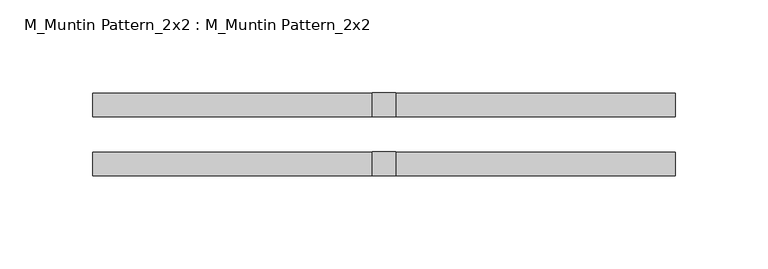
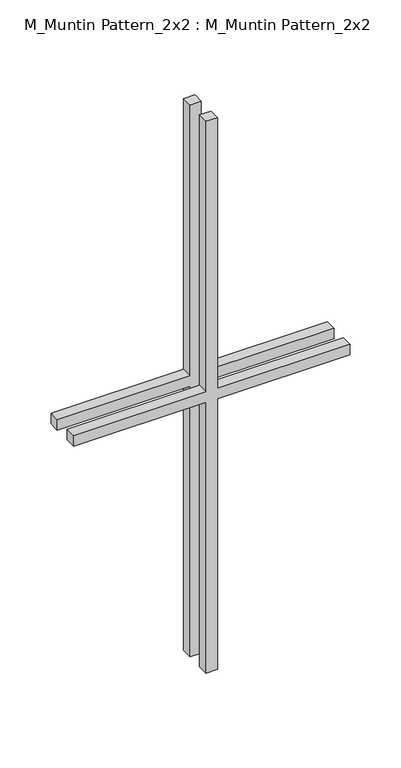
"""IFC4 building model written with IfcOpenShell, lengths in millimetres: proxy geometry, M_Muntin Pattern_2x2 : M_Muntin Pattern_2x2."""

from ifc_helpers import new_model, si_unit, frame, origin, place, context, project, spatial, polyline, outline, extrude, source, transform, mapped, element, save


def m_muntin_pattern_2x2_m_muntin_pattern_2x2_c959817e(model_context):
    return source(origin(), model_context, "Body", "SweptSolid", [
        extrude(outline(polyline([(336.5, -6.35), (336.5, -156.6333333), (323.8, -156.6333333), (323.8, -6.35), (0.0, -6.35), (0.0, 6.35), (323.8, 6.35), (323.8, 156.6333333), (336.5, 156.6333333), (336.5, 6.35), (660.3, 6.35), (660.3, -6.35), (336.5, -6.35)])), frame((0.0, 9.525, 0.0), z_axis=(0.0, 1.0, 0.0), x_axis=(0.0, 0.0, 1.0)), (0.0, 0.0, 1.0), 12.7),
        extrude(outline(polyline([(336.5, -6.35), (336.5, -156.6333333), (323.8, -156.6333333), (323.8, -6.35), (0.0, -6.35), (0.0, 6.35), (323.8, 6.35), (323.8, 156.6333333), (336.5, 156.6333333), (336.5, 6.35), (660.3, 6.35), (660.3, -6.35), (336.5, -6.35)])), frame((0.0, -22.225, 0.0), z_axis=(0.0, 1.0, 0.0), x_axis=(0.0, 0.0, 1.0)), (0.0, 0.0, 1.0), 12.7),
    ])


if __name__ == "__main__":
    model = new_model("IFC4")
    model_context = context("Model", 3, world=origin())
    ifc_project = project(units=[si_unit("LENGTHUNIT", "METRE", prefix="MILLI")], contexts=[model_context])
    site = spatial("IfcSite", under=ifc_project)
    building = spatial("IfcBuilding", under=site)
    placement = place(None, origin())
    m_muntin_pattern_2x2_m_muntin_pattern_2x2_shape = m_muntin_pattern_2x2_m_muntin_pattern_2x2_c959817e(model_context)
    element("IfcBuildingElementProxy", 1, Name="M_Muntin Pattern_2x2 : M_Muntin Pattern_2x2", ObjectType="M_Muntin Pattern_2x2 : M_Muntin Pattern_2x2", at=placement, inside=building, context=model_context, shape_type="MappedRepresentation", body=[
        mapped(m_muntin_pattern_2x2_m_muntin_pattern_2x2_shape, transform((0.0, 0.0, 0.0), x_axis=(1.0, 0.0, 0.0), y_axis=(0.0, 1.0, 0.0), z_axis=(0.0, 0.0, 1.0))),
    ])
    save(model, "model.ifc")

# Revit data of these elements
# Type "M_Muntin Pattern_2x2 : M_Muntin Pattern_2x2"
#   Width [instance default] = 3' - 11.24409"
#   Thickness = 0' - 0 1/2"
#   Height [instance default] = 3' - 11.24409"
#   Distance = 0' - 0 3/4"
#   Interior Material [instance default] = none
#   Exterior Material [instance default] = none
#   Default Elevation = 0
# Element 1 (IfcBuildingElementProxy, "M_Muntin Pattern_2x2 : M_Muntin Pattern_2x2")
#   Width = 1' - 0.33333"
#   Height = 2' - 1.99606"
#   Interior Material = Wood - Stained
#   Exterior Material = Clad - White
#   Materials on its faces: "Clad - White", "Wood - Stained"
# Materials
#   "Clad - White": class "Wood", colour RGB 242 242 238, transparency 0, Cost = 0
#   "Wood - Stained": class "Wood", colour RGB 227 170 128, transparency 0, Cost = 0
